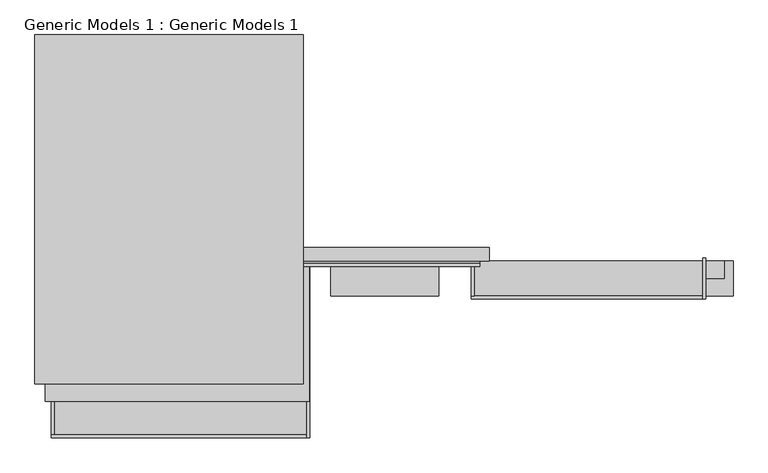
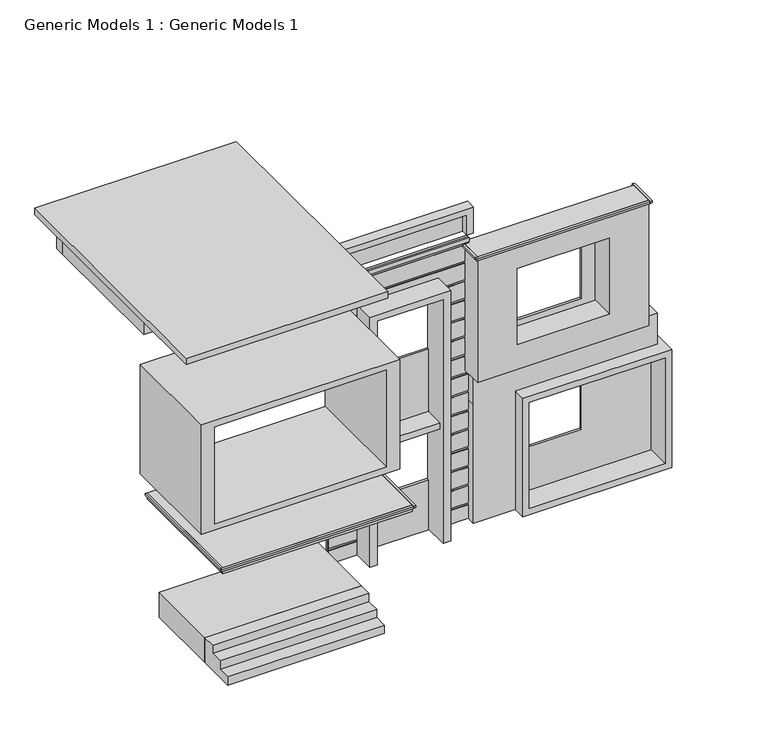
"""IFC4 building model written with IfcOpenShell, lengths in millimetres: proxy geometry, Generic Models 1 : Generic Models 1."""

from ifc_helpers import new_model, si_unit, frame, origin, origin_with_axes, place, context, project, spatial, polyline, outline, extrude, faceted_brep, source, transform, mapped, element, save


def generic_models_1_generic_models_1_556d1784(model_context):
    return source(origin(), model_context, "Body", "SolidModel", [
        extrude(outline(polyline([(-7879.4679297, 143.2196292), (-7879.4679297, -85.3803708), (-8317.6179297, -85.3803708), (-8317.6179297, 143.2196292), (-7879.4679297, 143.2196292)])), frame((0.0, 0.0, 7490.4399671), z_axis=(0.0, 0.0, 1.0), x_axis=(1.0, 0.0, 0.0)), (0.0, 0.0, 1.0), 202.0307064),
        extrude(outline(polyline([(-8031.8679297, 144.1522509), (-8031.8679297, 3685.9303652), (-7879.4679297, 3685.9303652), (-7879.4679297, 144.1522509), (-8031.8679297, 144.1522509)])), frame((0.0, 0.0, 6858.0), z_axis=(0.0, 0.0, 1.0), x_axis=(1.0, 0.0, 0.0)), (0.0, 0.0, 1.0), 834.4706735),
        extrude(outline(polyline([(-9568.5679297, 3838.3303652), (-9339.9679297, 3838.3303652), (-7879.4679297, 3838.3303652), (-7879.4679297, 3685.9303652), (-9339.9679297, 3685.9303652), (-9339.9679297, 3394.4196292), (-9568.5679297, 3394.4196292), (-11930.7679297, 3394.4196292), (-11930.7679297, 143.2196292), (-12159.3679297, 143.2196292), (-12159.3679297, 3394.4196292), (-12159.3679297, 3623.0196292), (-9568.5679297, 3623.0196292), (-9568.5679297, 3838.3303652)])), frame((0.0, 0.0, 6858.0), z_axis=(0.0, 0.0, 1.0), x_axis=(1.0, 0.0, 0.0)), (0.0, 0.0, 1.0), 834.4706735),
        extrude(outline(polyline([(-7879.4679297, -2224.2989686), (-12540.3679297, -2224.2989686), (-12540.3679297, 3838.3303652), (-7879.4679297, 3838.3303652), (-7879.4679297, -2224.2989686)])), frame((0.0, 0.0, 7692.4706735), z_axis=(0.0, 0.0, 1.0), x_axis=(1.0, 0.0, 0.0)), (0.0, 0.0, 1.0), 152.4),
        extrude(outline(polyline([(-8063.6179297, 143.2196292), (-4812.4179297, 143.2196292), (-4812.4179297, 79.7196292), (-8063.6179297, 79.7196292), (-8063.6179297, 143.2196292)])), frame((0.0, 0.0, 6858.0), z_axis=(0.0, 0.0, 1.0), x_axis=(1.0, 0.0, 0.0)), (0.0, 0.0, 1.0), 486.1154283),
        extrude(outline(polyline([(6858.0, -8063.6179297), (7344.1154283, -8063.6179297), (7344.1154283, -4812.4179297), (6858.0, -4812.4179297), (6858.0, -4660.0179297), (7496.5154283, -4660.0179297), (7496.5154283, -8298.5679297), (6858.0, -8298.5679297), (6858.0, -8063.6179297)])), frame((0.0, -85.3803708, 0.0), z_axis=(0.0, 1.0, 0.0), x_axis=(0.0, 0.0, 1.0)), (0.0, 0.0, 1.0), 228.6),
        extrude(outline(polyline([(-900.8179297, -34.5803708), (-900.8179297, -745.7803708), (-951.6179297, -745.7803708), (-951.6179297, -34.5803708), (-900.8179297, -34.5803708)])), frame((0.0, 0.0, 6680.2), z_axis=(0.0, 0.0, 1.0), x_axis=(1.0, 0.0, 0.0)), (0.0, 0.0, 1.0), 50.8),
        extrude(outline(polyline([(-4964.8179297, -694.9803708), (-4964.8179297, -186.9803708), (-4914.0179297, -186.9803708), (-4914.0179297, -694.9803708), (-4964.8179297, -694.9803708)])), frame((0.0, 0.0, 6680.2), z_axis=(0.0, 0.0, 1.0), x_axis=(1.0, 0.0, 0.0)), (0.0, 0.0, 1.0), 50.8),
        extrude(outline(polyline([(-951.6179297, -745.7803708), (-4964.8179297, -745.7803708), (-4964.8179297, -694.9803708), (-951.6179297, -694.9803708), (-951.6179297, -745.7803708)])), frame((0.0, 0.0, 6680.2), z_axis=(0.0, 0.0, 1.0), x_axis=(1.0, 0.0, 0.0)), (0.0, 0.0, 1.0), 50.8),
        extrude(outline(polyline([(4267.2, -4018.6679297), (4267.2, -1885.0679297), (6121.4, -1885.0679297), (6121.4, -4018.6679297), (4267.2, -4018.6679297)]), holes=[polyline([(4419.6, -3713.8679297), (5969.0, -3713.8679297), (5969.0, -2189.8679297), (4419.6, -2189.8679297), (4419.6, -3713.8679297)])]), frame((0.0, -136.1803708, 0.0), z_axis=(0.0, 1.0, 0.0), x_axis=(0.0, 0.0, 1.0)), (0.0, 0.0, 1.0), 50.8),
        extrude(outline(polyline([(1219.2, -2189.8679297), (1219.2, -3713.8679297), (152.4, -3713.8679297), (152.4, -2189.8679297), (152.4, -576.9679297), (2743.2, -576.9679297), (2743.2, -2189.8679297), (1219.2, -2189.8679297)])), frame((0.0, -136.1803708, 0.0), z_axis=(0.0, 1.0, 0.0), x_axis=(0.0, 0.0, 1.0)), (0.0, 0.0, 1.0), 50.8),
        extrude(outline(polyline([(3657.6, -4914.0179297), (3657.6, -951.6179297), (6731.0, -951.6179297), (6731.0, -4914.0179297), (3657.6, -4914.0179297)]), holes=[polyline([(6121.4, -1866.0179297), (4267.2, -1866.0179297), (4267.2, -3999.6179297), (6121.4, -3999.6179297), (6121.4, -1866.0179297)])]), frame((0.0, -694.9803708, 0.0), z_axis=(0.0, 1.0, 0.0), x_axis=(0.0, 0.0, 1.0)), (0.0, 0.0, 1.0), 609.6),
        extrude(outline(polyline([(2895.6, -4836.3153615), (0.0, -4836.3153615), (0.0, -3866.2679297), (2895.6, -3866.2679297), (2895.6, -576.9679297), (3657.6, -576.9679297), (3657.6, -4836.3153615), (2895.6, -4836.3153615)])), frame((0.0, -390.1803708, 0.0), z_axis=(0.0, 1.0, 0.0), x_axis=(0.0, 0.0, 1.0)), (0.0, 0.0, 1.0), 304.8),
        extrude(outline(polyline([(0.0, -3866.2679297), (0.0, -424.5679297), (2895.6, -424.5679297), (2895.6, -3866.2679297), (0.0, -3866.2679297)]), holes=[polyline([(152.4, -3713.8679297), (2743.2, -3713.8679297), (2743.2, -576.9679297), (152.4, -576.9679297), (152.4, -3713.8679297)])]), frame((0.0, -694.9803708, 0.0), z_axis=(0.0, 1.0, 0.0), x_axis=(0.0, 0.0, 1.0)), (0.0, 0.0, 1.0), 609.6),
        faceted_brep([(-8063.6179297, -186.9803708, 0.0), (-7409.7974608, -186.9803708, 0.0), (-7409.7974608, -186.9803708, 333.7154283), (-8063.6179297, -186.9803708, 333.7154283), (-7409.7974608, -186.9803708, 6121.4), (-5535.77405, -186.9803708, 6121.4), (-5535.77405, -186.9803708, 5870.9154283), (-4817.2653615, -186.9803708, 5870.9154283), (-4817.2653615, -186.9803708, 6277.3154283), (-8063.6179297, -186.9803708, 6277.3154283), (-8063.6179297, -186.9803708, 5870.9154283), (-7409.7974608, -186.9803708, 5870.9154283), (-5535.77405, -186.9803708, 0.0), (-4817.2653615, -186.9803708, 0.0), (-4817.2653615, -186.9803708, 333.7154283), (-5535.77405, -186.9803708, 333.7154283), (-4817.2653615, -186.9803708, 6858.0), (-8063.6179297, -186.9803708, 6858.0), (-8063.6179297, -186.9803708, 6759.9154283), (-4817.2653615, -186.9803708, 6759.9154283), (-7409.7974608, -186.9803708, 384.5154283), (-7409.7974608, -186.9803708, 790.9154283), (-8063.6179297, -186.9803708, 790.9154283), (-8063.6179297, -186.9803708, 384.5154283), (-7409.7974608, -186.9803708, 841.7154283), (-7409.7974608, -186.9803708, 1248.1154283), (-8063.6179297, -186.9803708, 1248.1154283), (-8063.6179297, -186.9803708, 841.7154283), (-7409.7974608, -186.9803708, 1298.9154283), (-7409.7974608, -186.9803708, 1705.3154283), (-8063.6179297, -186.9803708, 1705.3154283), (-8063.6179297, -186.9803708, 1298.9154283), (-7409.7974608, -186.9803708, 1756.1154283), (-7409.7974608, -186.9803708, 2162.5154283), (-8063.6179297, -186.9803708, 2162.5154283), (-8063.6179297, -186.9803708, 1756.1154283), (-7409.7974608, -186.9803708, 2213.3154283), (-7409.7974608, -186.9803708, 2619.7154283), (-8063.6179297, -186.9803708, 2619.7154283), (-8063.6179297, -186.9803708, 2213.3154283), (-7409.7974608, -186.9803708, 2670.5154283), (-7409.7974608, -186.9803708, 3076.9154283), (-7749.8885054, -186.9803708, 3076.9154283), (-7749.8885054, -186.9803708, 3127.7154283), (-7409.7974608, -186.9803708, 3127.7154283), (-7409.7974608, -186.9803708, 3534.1154283), (-7860.4179297, -186.9803708, 3534.1154283), (-7860.4179297, -186.9803708, 3584.9154283), (-7409.7974608, -186.9803708, 3584.9154283), (-7409.7974608, -186.9803708, 3991.3154283), (-8063.6179297, -186.9803708, 3991.3154283), (-8063.6179297, -186.9803708, 2670.5154283), (-7409.7974608, -186.9803708, 4042.1154283), (-7409.7974608, -186.9803708, 4448.5154283), (-8063.6179297, -186.9803708, 4448.5154283), (-8063.6179297, -186.9803708, 4042.1154283), (-7409.7974608, -186.9803708, 4499.3154283), (-7409.7974608, -186.9803708, 4905.7154283), (-8063.6179297, -186.9803708, 4905.7154283), (-8063.6179297, -186.9803708, 4499.3154283), (-7409.7974608, -186.9803708, 4956.5154283), (-7409.7974608, -186.9803708, 5362.9154283), (-8063.6179297, -186.9803708, 5362.9154283), (-8063.6179297, -186.9803708, 4956.5154283), (-7409.7974608, -186.9803708, 5413.7154283), (-7409.7974608, -186.9803708, 5820.1154283), (-8063.6179297, -186.9803708, 5820.1154283), (-8063.6179297, -186.9803708, 5413.7154283), (-5535.77405, -186.9803708, 790.9154283), (-5535.77405, -186.9803708, 384.5154283), (-4817.2653615, -186.9803708, 384.5154283), (-4817.2653615, -186.9803708, 790.9154283), (-5535.77405, -186.9803708, 1248.1154283), (-5535.77405, -186.9803708, 841.7154283), (-4817.2653615, -186.9803708, 841.7154283), (-4817.2653615, -186.9803708, 1248.1154283), (-5535.77405, -186.9803708, 1705.3154283), (-5535.77405, -186.9803708, 1298.9154283), (-4817.2653615, -186.9803708, 1298.9154283), (-4817.2653615, -186.9803708, 1705.3154283), (-5535.77405, -186.9803708, 2162.5154283), (-5535.77405, -186.9803708, 1756.1154283), (-4817.2653615, -186.9803708, 1756.1154283), (-4817.2653615, -186.9803708, 2162.5154283), (-5535.77405, -186.9803708, 2619.7154283), (-5535.77405, -186.9803708, 2213.3154283), (-4817.2653615, -186.9803708, 2213.3154283), (-4817.2653615, -186.9803708, 2619.7154283), (-5535.77405, -186.9803708, 3076.9154283), (-5535.77405, -186.9803708, 2670.5154283), (-4817.2653615, -186.9803708, 2670.5154283), (-4817.2653615, -186.9803708, 3076.9154283), (-5535.77405, -186.9803708, 3534.1154283), (-5535.77405, -186.9803708, 3127.7154283), (-4817.2653615, -186.9803708, 3127.7154283), (-4817.2653615, -186.9803708, 3534.1154283), (-5535.77405, -186.9803708, 3991.3154283), (-5535.77405, -186.9803708, 3584.9154283), (-4817.2653615, -186.9803708, 3584.9154283), (-4817.2653615, -186.9803708, 3991.3154283), (-5535.77405, -186.9803708, 4448.5154283), (-5535.77405, -186.9803708, 4042.1154283), (-4817.2653615, -186.9803708, 4042.1154283), (-4817.2653615, -186.9803708, 4448.5154283), (-5535.77405, -186.9803708, 4905.7154283), (-5535.77405, -186.9803708, 4499.3154283), (-4817.2653615, -186.9803708, 4499.3154283), (-4817.2653615, -186.9803708, 4905.7154283), (-5535.77405, -186.9803708, 5362.9154283), (-5535.77405, -186.9803708, 4956.5154283), (-4817.2653615, -186.9803708, 4956.5154283), (-4817.2653615, -186.9803708, 5362.9154283), (-5535.77405, -186.9803708, 5820.1154283), (-5535.77405, -186.9803708, 5413.7154283), (-4817.2653615, -186.9803708, 5413.7154283), (-4817.2653615, -186.9803708, 5820.1154283), (-4817.2653615, -186.9803708, 6328.1154283), (-4817.2653615, -186.9803708, 6709.1154283), (-8063.6179297, -186.9803708, 6709.1154283), (-8063.6179297, -186.9803708, 6328.1154283), (-8063.6179297, -136.1803708, 0.0), (-8063.6179297, -136.1803708, 6858.0), (-4817.2653615, -136.1803708, 6858.0), (-4817.2653615, -136.1803708, 0.0), (-5535.77405, -136.1803708, 0.0), (-5535.77405, -136.1803708, 6121.4), (-7409.7974608, -136.1803708, 6121.4), (-7409.7974608, -136.1803708, 0.0), (-7409.7974608, -174.2803708, 5870.9154283), (-7409.7974608, -174.2803708, 5820.1154283), (-7409.7974608, -174.2803708, 5413.7154283), (-7409.7974608, -174.2803708, 5362.9154283), (-7409.7974608, -174.2803708, 4956.5154283), (-7409.7974608, -174.2803708, 4905.7154283), (-7409.7974608, -174.2803708, 4499.3154283), (-7409.7974608, -174.2803708, 4448.5154283), (-7409.7974608, -174.2803708, 4042.1154283), (-7409.7974608, -174.2803708, 3991.3154283), (-7409.7974608, -174.2803708, 3584.9154283), (-7409.7974608, -174.2803708, 3534.1154283), (-7409.7974608, -174.2803708, 3127.7154283), (-7409.7974608, -174.2803708, 3076.9154283), (-7409.7974608, -174.2803708, 2670.5154283), (-7409.7974608, -174.2803708, 2619.7154283), (-7409.7974608, -174.2803708, 2213.3154283), (-7409.7974608, -174.2803708, 2162.5154283), (-7409.7974608, -174.2803708, 1756.1154283), (-7409.7974608, -174.2803708, 1705.3154283), (-7409.7974608, -174.2803708, 1298.9154283), (-7409.7974608, -174.2803708, 1248.1154283), (-7409.7974608, -174.2803708, 841.7154283), (-7409.7974608, -174.2803708, 790.9154283), (-7409.7974608, -174.2803708, 384.5154283), (-7409.7974608, -174.2803708, 333.7154283), (-5535.77405, -174.2803708, 333.7154283), (-5535.77405, -174.2803708, 384.5154283), (-5535.77405, -174.2803708, 790.9154283), (-5535.77405, -174.2803708, 841.7154283), (-5535.77405, -174.2803708, 1248.1154283), (-5535.77405, -174.2803708, 1298.9154283), (-5535.77405, -174.2803708, 1705.3154283), (-5535.77405, -174.2803708, 1756.1154283), (-5535.77405, -174.2803708, 2162.5154283), (-5535.77405, -174.2803708, 2213.3154283), (-5535.77405, -174.2803708, 2619.7154283), (-5535.77405, -174.2803708, 2670.5154283), (-5535.77405, -174.2803708, 3076.9154283), (-5535.77405, -174.2803708, 3127.7154283), (-5535.77405, -174.2803708, 3534.1154283), (-5535.77405, -174.2803708, 3584.9154283), (-5535.77405, -174.2803708, 3991.3154283), (-5535.77405, -174.2803708, 4042.1154283), (-5535.77405, -174.2803708, 4448.5154283), (-5535.77405, -174.2803708, 4499.3154283), (-5535.77405, -174.2803708, 4905.7154283), (-5535.77405, -174.2803708, 4956.5154283), (-5535.77405, -174.2803708, 5362.9154283), (-5535.77405, -174.2803708, 5413.7154283), (-5535.77405, -174.2803708, 5820.1154283), (-5535.77405, -174.2803708, 5870.9154283), (-4817.2653615, -174.2803708, 6759.9154283), (-4817.2653615, -174.2803708, 6709.1154283), (-4817.2653615, -174.2803708, 6328.1154283), (-4817.2653615, -174.2803708, 6277.3154283), (-4817.2653615, -174.2803708, 5870.9154283), (-4817.2653615, -174.2803708, 5820.1154283), (-4817.2653615, -174.2803708, 5413.7154283), (-4817.2653615, -174.2803708, 5362.9154283), (-4817.2653615, -174.2803708, 4956.5154283), (-4817.2653615, -174.2803708, 4905.7154283), (-4817.2653615, -174.2803708, 4499.3154283), (-4817.2653615, -174.2803708, 4448.5154283), (-4817.2653615, -174.2803708, 4042.1154283), (-4817.2653615, -174.2803708, 3991.3154283), (-4817.2653615, -174.2803708, 3584.9154283), (-4817.2653615, -174.2803708, 3534.1154283), (-4817.2653615, -174.2803708, 3127.7154283), (-4817.2653615, -174.2803708, 3076.9154283), (-4817.2653615, -174.2803708, 2670.5154283), (-4817.2653615, -174.2803708, 2619.7154283), (-4817.2653615, -174.2803708, 2213.3154283), (-4817.2653615, -174.2803708, 2162.5154283), (-4817.2653615, -174.2803708, 1756.1154283), (-4817.2653615, -174.2803708, 1705.3154283), (-4817.2653615, -174.2803708, 1298.9154283), (-4817.2653615, -174.2803708, 1248.1154283), (-4817.2653615, -174.2803708, 841.7154283), (-4817.2653615, -174.2803708, 790.9154283), (-4817.2653615, -174.2803708, 384.5154283), (-4817.2653615, -174.2803708, 333.7154283), (-8063.6179297, -174.2803708, 333.7154283), (-8063.6179297, -174.2803708, 384.5154283), (-8063.6179297, -174.2803708, 790.9154283), (-8063.6179297, -174.2803708, 841.7154283), (-8063.6179297, -174.2803708, 1248.1154283), (-8063.6179297, -174.2803708, 1298.9154283), (-8063.6179297, -174.2803708, 1705.3154283), (-8063.6179297, -174.2803708, 1756.1154283), (-8063.6179297, -174.2803708, 2162.5154283), (-8063.6179297, -174.2803708, 2213.3154283), (-8063.6179297, -174.2803708, 2619.7154283), (-8063.6179297, -174.2803708, 2670.5154283), (-8063.6179297, -174.2803708, 3991.3154283), (-8063.6179297, -174.2803708, 4042.1154283), (-8063.6179297, -174.2803708, 4448.5154283), (-8063.6179297, -174.2803708, 4499.3154283), (-8063.6179297, -174.2803708, 4905.7154283), (-8063.6179297, -174.2803708, 4956.5154283), (-8063.6179297, -174.2803708, 5362.9154283), (-8063.6179297, -174.2803708, 5413.7154283), (-8063.6179297, -174.2803708, 5820.1154283), (-8063.6179297, -174.2803708, 5870.9154283), (-8063.6179297, -174.2803708, 6277.3154283), (-8063.6179297, -174.2803708, 6328.1154283), (-8063.6179297, -174.2803708, 6709.1154283), (-8063.6179297, -174.2803708, 6759.9154283), (-7749.8885054, -174.2803708, 3127.7154283), (-7749.8885054, -174.2803708, 3076.9154283), (-7860.4179297, -174.2803708, 3584.9154283), (-7860.4179297, -174.2803708, 3534.1154283)], [[[0, 1, 2, 3]], [[4, 5, 6, 7, 8, 9, 10, 11]], [[12, 13, 14, 15]], [[16, 17, 18, 19]], [[20, 21, 22, 23]], [[24, 25, 26, 27]], [[28, 29, 30, 31]], [[32, 33, 34, 35]], [[36, 37, 38, 39]], [[40, 41, 42, 43, 44, 45, 46, 47, 48, 49, 50, 51]], [[52, 53, 54, 55]], [[56, 57, 58, 59]], [[60, 61, 62, 63]], [[64, 65, 66, 67]], [[68, 69, 70, 71]], [[72, 73, 74, 75]], [[76, 77, 78, 79]], [[80, 81, 82, 83]], [[84, 85, 86, 87]], [[88, 89, 90, 91]], [[92, 93, 94, 95]], [[96, 97, 98, 99]], [[100, 101, 102, 103]], [[104, 105, 106, 107]], [[108, 109, 110, 111]], [[112, 113, 114, 115]], [[116, 117, 118, 119]], [[120, 121, 122, 123, 124, 125, 126, 127]], [[1, 0, 120, 127]], [[127, 126, 4, 11, 128, 129, 65, 64, 130, 131, 61, 60, 132, 133, 57, 56, 134, 135, 53, 52, 136, 137, 49, 48, 138, 139, 45, 44, 140, 141, 41, 40, 142, 143, 37, 36, 144, 145, 33, 32, 146, 147, 29, 28, 148, 149, 25, 24, 150, 151, 21, 20, 152, 153, 2, 1]], [[5, 4, 126, 125]], [[125, 124, 12, 15, 154, 155, 69, 68, 156, 157, 73, 72, 158, 159, 77, 76, 160, 161, 81, 80, 162, 163, 85, 84, 164, 165, 89, 88, 166, 167, 93, 92, 168, 169, 97, 96, 170, 171, 101, 100, 172, 173, 105, 104, 174, 175, 109, 108, 176, 177, 113, 112, 178, 179, 6, 5]], [[13, 12, 124, 123]], [[123, 122, 16, 19, 180, 181, 117, 116, 182, 183, 8, 7, 184, 185, 115, 114, 186, 187, 111, 110, 188, 189, 107, 106, 190, 191, 103, 102, 192, 193, 99, 98, 194, 195, 95, 94, 196, 197, 91, 90, 198, 199, 87, 86, 200, 201, 83, 82, 202, 203, 79, 78, 204, 205, 75, 74, 206, 207, 71, 70, 208, 209, 14, 13]], [[17, 16, 122, 121]], [[121, 120, 0, 3, 210, 211, 23, 22, 212, 213, 27, 26, 214, 215, 31, 30, 216, 217, 35, 34, 218, 219, 39, 38, 220, 221, 51, 50, 222, 223, 55, 54, 224, 225, 59, 58, 226, 227, 63, 62, 228, 229, 67, 66, 230, 231, 10, 9, 232, 233, 119, 118, 234, 235, 18, 17]], [[152, 211, 210, 153]], [[150, 213, 212, 151]], [[148, 215, 214, 149]], [[146, 217, 216, 147]], [[144, 219, 218, 145]], [[142, 221, 220, 143]], [[140, 236, 237, 141]], [[138, 238, 239, 139]], [[136, 223, 222, 137]], [[134, 225, 224, 135]], [[132, 227, 226, 133]], [[130, 229, 228, 131]], [[128, 231, 230, 129]], [[182, 233, 232, 183]], [[180, 235, 234, 181]], [[208, 155, 154, 209]], [[206, 157, 156, 207]], [[204, 159, 158, 205]], [[202, 161, 160, 203]], [[200, 163, 162, 201]], [[198, 165, 164, 199]], [[196, 167, 166, 197]], [[194, 169, 168, 195]], [[192, 171, 170, 193]], [[190, 173, 172, 191]], [[188, 175, 174, 189]], [[186, 177, 176, 187]], [[184, 179, 178, 185]], [[153, 210, 3, 2]], [[211, 152, 20, 23]], [[151, 212, 22, 21]], [[213, 150, 24, 27]], [[149, 214, 26, 25]], [[215, 148, 28, 31]], [[147, 216, 30, 29]], [[217, 146, 32, 35]], [[145, 218, 34, 33]], [[219, 144, 36, 39]], [[143, 220, 38, 37]], [[221, 142, 40, 51]], [[141, 237, 42, 41]], [[237, 236, 43, 42]], [[236, 140, 44, 43]], [[139, 239, 46, 45]], [[239, 238, 47, 46]], [[238, 138, 48, 47]], [[137, 222, 50, 49]], [[223, 136, 52, 55]], [[135, 224, 54, 53]], [[225, 134, 56, 59]], [[133, 226, 58, 57]], [[227, 132, 60, 63]], [[131, 228, 62, 61]], [[229, 130, 64, 67]], [[129, 230, 66, 65]], [[231, 128, 11, 10]], [[183, 232, 9, 8]], [[233, 182, 116, 119]], [[181, 234, 118, 117]], [[235, 180, 19, 18]], [[209, 154, 15, 14]], [[155, 208, 70, 69]], [[207, 156, 68, 71]], [[157, 206, 74, 73]], [[205, 158, 72, 75]], [[159, 204, 78, 77]], [[203, 160, 76, 79]], [[161, 202, 82, 81]], [[201, 162, 80, 83]], [[163, 200, 86, 85]], [[199, 164, 84, 87]], [[165, 198, 90, 89]], [[197, 166, 88, 91]], [[167, 196, 94, 93]], [[195, 168, 92, 95]], [[169, 194, 98, 97]], [[193, 170, 96, 99]], [[171, 192, 102, 101]], [[191, 172, 100, 103]], [[173, 190, 106, 105]], [[189, 174, 104, 107]], [[175, 188, 110, 109]], [[187, 176, 108, 111]], [[177, 186, 114, 113]], [[185, 178, 112, 115]], [[179, 184, 7, 6]]]),
        extrude(outline(polyline([(0.0, -8063.6179297), (0.0, -7238.1179297), (6121.4, -7238.1179297), (6121.4, -5535.77405), (0.0, -5535.77405), (0.0, -4817.2653615), (6858.0, -4817.2653615), (6858.0, -8063.6179297), (0.0, -8063.6179297)])), frame((0.0, -136.1803708, 0.0), z_axis=(0.0, 1.0, 0.0), x_axis=(0.0, 0.0, 1.0)), (0.0, 0.0, 1.0), 50.8),
        extrude(outline(polyline([(5969.0, -5714.1179297), (0.0, -5714.1179297), (0.0, -5535.77405), (6121.4, -5535.77405), (6121.4, -7409.7974608), (0.0, -7409.7974608), (0.0, -7238.1179297), (5969.0, -7238.1179297), (5969.0, -5714.1179297)])), frame((0.0, -694.9803708, 0.0), z_axis=(0.0, 1.0, 0.0), x_axis=(0.0, 0.0, 1.0)), (0.0, 0.0, 1.0), 609.6),
        faceted_brep([(-12362.5679297, -2529.0989686, 6332.6526577), (-12362.5679297, -2529.0989686, 3657.6), (-7777.8679297, -2529.0989686, 3657.6), (-7777.8679297, -2529.0989686, 6332.6526577), (-12057.7679297, -2529.0989686, 3810.0), (-12057.7679297, -2529.0989686, 6180.2526577), (-8082.6679297, -2529.0989686, 6180.2526577), (-8082.6679297, -2529.0989686, 3810.0), (-12362.5679297, -85.3803708, 6332.6526577), (-7777.8679297, -85.3803708, 6332.6526577), (-7777.8679297, -85.3803708, 3657.6), (-12362.5679297, -85.3803708, 3657.6), (-12057.7679297, -85.3803708, 3810.0), (-8082.6679297, -85.3803708, 3810.0), (-8082.6679297, -85.3803708, 6180.2526577), (-12057.7679297, -85.3803708, 6180.2526577), (-7777.8679297, -174.2803708, 4042.1154283), (-7777.8679297, -174.2803708, 3991.3154283), (-7777.8679297, -186.9803708, 3991.3154283), (-7777.8679297, -186.9803708, 4042.1154283), (-7777.8679297, -174.2803708, 4499.3154283), (-7777.8679297, -174.2803708, 4448.5154283), (-7777.8679297, -186.9803708, 4448.5154283), (-7777.8679297, -186.9803708, 4499.3154283), (-7777.8679297, -174.2803708, 4956.5154283), (-7777.8679297, -174.2803708, 4905.7154283), (-7777.8679297, -186.9803708, 4905.7154283), (-7777.8679297, -186.9803708, 4956.5154283), (-7777.8679297, -174.2803708, 5413.7154283), (-7777.8679297, -174.2803708, 5362.9154283), (-7777.8679297, -186.9803708, 5362.9154283), (-7777.8679297, -186.9803708, 5413.7154283), (-7777.8679297, -174.2803708, 5870.9154283), (-7777.8679297, -174.2803708, 5820.1154283), (-7777.8679297, -186.9803708, 5820.1154283), (-7777.8679297, -186.9803708, 5870.9154283), (-7777.8679297, -174.2803708, 6328.1154283), (-7777.8679297, -174.2803708, 6277.3154283), (-7777.8679297, -186.9803708, 6277.3154283), (-7777.8679297, -186.9803708, 6328.1154283), (-8063.6179297, -174.2803708, 6328.1154283), (-8063.6179297, -174.2803708, 6277.3154283), (-8063.6179297, -174.2803708, 4042.1154283), (-8063.6179297, -174.2803708, 3991.3154283), (-8063.6179297, -174.2803708, 4499.3154283), (-8063.6179297, -174.2803708, 4448.5154283), (-8063.6179297, -174.2803708, 4956.5154283), (-8063.6179297, -174.2803708, 4905.7154283), (-8063.6179297, -174.2803708, 5413.7154283), (-8063.6179297, -174.2803708, 5362.9154283), (-8063.6179297, -174.2803708, 5870.9154283), (-8063.6179297, -174.2803708, 5820.1154283), (-8063.6179297, -186.9803708, 6277.3154283), (-8063.6179297, -186.9803708, 6328.1154283), (-8063.6179297, -186.9803708, 3991.3154283), (-8063.6179297, -186.9803708, 4042.1154283), (-8063.6179297, -186.9803708, 4448.5154283), (-8063.6179297, -186.9803708, 4499.3154283), (-8063.6179297, -186.9803708, 4905.7154283), (-8063.6179297, -186.9803708, 4956.5154283), (-8063.6179297, -186.9803708, 5362.9154283), (-8063.6179297, -186.9803708, 5413.7154283), (-8063.6179297, -186.9803708, 5820.1154283), (-8063.6179297, -186.9803708, 5870.9154283)], [[[0, 1, 2, 3], [4, 5, 6, 7]], [[8, 9, 10, 11], [12, 13, 14, 15]], [[5, 4, 12, 15]], [[6, 5, 15, 14]], [[7, 6, 14, 13]], [[4, 7, 13, 12]], [[1, 0, 8, 11]], [[2, 1, 11, 10]], [[3, 2, 10, 9], [16, 17, 18, 19], [20, 21, 22, 23], [24, 25, 26, 27], [28, 29, 30, 31], [32, 33, 34, 35], [36, 37, 38, 39]], [[0, 3, 9, 8]], [[40, 41, 37, 36]], [[42, 43, 17, 16]], [[44, 45, 21, 20]], [[46, 47, 25, 24]], [[48, 49, 29, 28]], [[50, 51, 33, 32]], [[52, 53, 39, 38]], [[54, 55, 19, 18]], [[56, 57, 23, 22]], [[58, 59, 27, 26]], [[60, 61, 31, 30]], [[62, 63, 35, 34]], [[43, 54, 18, 17]], [[55, 42, 16, 19]], [[45, 56, 22, 21]], [[57, 44, 20, 23]], [[47, 58, 26, 25]], [[59, 46, 24, 27]], [[49, 60, 30, 29]], [[61, 48, 28, 31]], [[51, 62, 34, 33]], [[63, 50, 32, 35]], [[41, 52, 38, 37]], [[41, 40, 53, 52]], [[53, 40, 36, 39]], [[43, 42, 55, 54]], [[45, 44, 57, 56]], [[47, 46, 59, 58]], [[49, 48, 61, 60]], [[51, 50, 63, 62]]]),
        extrude(outline(polyline([(-7768.9385054, -85.3803708), (-7768.9385054, -3158.8511799), (-7819.7385054, -3158.8511799), (-7819.7385054, -85.3803708), (-7768.9385054, -85.3803708)])), frame((0.0, 0.0, 3086.5208873), z_axis=(0.0, 0.0, 1.0), x_axis=(1.0, 0.0, 0.0)), (0.0, 0.0, 1.0), 50.8),
        extrude(outline(polyline([(-5733.1679297, -593.3803708), (-7257.1679297, -593.3803708), (-7257.1679297, -136.1803708), (-5733.1679297, -136.1803708), (-5733.1679297, -593.3803708)])), frame((0.0, 0.0, 2743.2), z_axis=(0.0, 0.0, 1.0), x_axis=(1.0, 0.0, 0.0)), (0.0, 0.0, 1.0), 152.4),
        extrude(outline(polyline([(-5733.1679297, -136.1803708), (-7257.1679297, -136.1803708), (-7257.1679297, -85.3803708), (-5733.1679297, -85.3803708), (-5733.1679297, -136.1803708)])), frame((0.0, 0.0, 2895.6), z_axis=(0.0, 0.0, 1.0), x_axis=(1.0, 0.0, 0.0)), (0.0, 0.0, 1.0), 1524.0),
        extrude(outline(polyline([(-5733.1679297, -136.1803708), (-7257.1679297, -136.1803708), (-7257.1679297, -85.3803708), (-5733.1679297, -85.3803708), (-5733.1679297, -136.1803708)])), origin_with_axes(), (0.0, 0.0, 1.0), 1219.2),
        extrude(outline(polyline([(-5714.1179297, -136.1803708), (-7238.1179297, -136.1803708), (-7238.1179297, -85.3803708), (-5714.1179297, -85.3803708), (-5714.1179297, -136.1803708)])), frame((0.0, 0.0, 2743.2), z_axis=(0.0, 0.0, 1.0), x_axis=(1.0, 0.0, 0.0)), (0.0, 0.0, 1.0), 152.4),
        extrude(outline(polyline([(-7819.7385054, -3158.8511799), (-12255.0398919, -3158.8511799), (-12255.0398919, -3108.0511799), (-7819.7385054, -3108.0511799), (-7819.7385054, -3158.8511799)])), frame((0.0, 0.0, 3086.5208873), z_axis=(0.0, 0.0, 1.0), x_axis=(1.0, 0.0, 0.0)), (0.0, 0.0, 1.0), 50.8),
        extrude(outline(polyline([(-12255.0398919, -3108.0511799), (-12255.0398919, -85.4511799), (-12204.2398919, -85.4511799), (-12204.2398919, -3108.0511799), (-12255.0398919, -3108.0511799)])), frame((0.0, 0.0, 3086.5208873), z_axis=(0.0, 0.0, 1.0), x_axis=(1.0, 0.0, 0.0)), (0.0, 0.0, 1.0), 50.8),
        extrude(outline(polyline([(-7819.7385054, -3108.0511799), (-12204.2398919, -3108.0511799), (-12204.2398919, -85.3803708), (-7819.7385054, -85.3803708), (-7819.7385054, -3108.0511799)])), frame((0.0, 0.0, 2984.9208873), z_axis=(0.0, 0.0, 1.0), x_axis=(1.0, 0.0, 0.0)), (0.0, 0.0, 1.0), 152.4),
        extrude(outline(polyline([(-1919.4989686, 609.6), (-1919.4989686, 0.0), (-2833.8989686, 0.0), (-2833.8989686, 203.2), (-2529.0989686, 203.2), (-2529.0989686, 406.4), (-2224.2989686, 406.4), (-2224.2989686, 609.6), (-1919.4989686, 609.6)])), frame((-11930.7679297, 0.0, 0.0), z_axis=(1.0, 0.0, 0.0), x_axis=(0.0, 1.0, 0.0)), (0.0, 0.0, 1.0), 3619.5),
        extrude(outline(polyline([(-8311.2679297, -1919.4989686), (-11930.7679297, -1919.4989686), (-11930.7679297, -85.3803708), (-8311.2679297, -85.3803708), (-8311.2679297, -1919.4989686)])), origin_with_axes(), (0.0, 0.0, 1.0), 609.6),
    ])


if __name__ == "__main__":
    model = new_model("IFC4")
    model_context = context("Model", 3, world=origin())
    ifc_project = project(units=[si_unit("LENGTHUNIT", "METRE", prefix="MILLI")], contexts=[model_context])
    site = spatial("IfcSite", under=ifc_project)
    building = spatial("IfcBuilding", under=site)
    placement = place(None, origin())
    generic_models_1_generic_models_1_shape = generic_models_1_generic_models_1_556d1784(model_context)
    element("IfcBuildingElementProxy", 1, Name="Generic Models 1 : Generic Models 1", ObjectType="Generic Models 1 : Generic Models 1", at=placement, inside=building, context=model_context, shape_type="MappedRepresentation", body=[
        mapped(generic_models_1_generic_models_1_shape, transform((0.0, 0.0, 0.0), x_axis=(1.0, 0.0, 0.0), y_axis=(0.0, 1.0, 0.0), z_axis=(0.0, 0.0, 1.0))),
    ])
    save(model, "model.ifc")

# Revit data of these elements
# Element 1 (IfcBuildingElementProxy, "Generic Models 1 : Generic Models 1")
#   Materials on its faces: "light ash colour", "Laminate, Ivory, Matte", "Gypsum Wall Board", "Ash colour", "door colour", "window brick", "Ash brick", "Earth", "Concrete, Lightweight"
# Materials
#   "light ash colour": class "Generic", colour RGB 120 120 120, transparency 0, Cost = 0
#   "Laminate, Ivory, Matte": class "Plastic", colour RGB 247 247 239, transparency 0, Description = "Plastic Laminate - Ivory, Matte", Cost = 0
#   "Gypsum Wall Board": class "Generic", colour RGB 127 127 127, transparency 0, Description = "Gypsum Wall Board", Cost = 0
#   "Ash colour": class "Generic", colour RGB 120 120 120, transparency 0, Cost = 0
#   "door colour": class "Generic", colour RGB 120 120 120, transparency 0, Cost = 0
#   "window brick": class "Generic", colour RGB 120 120 120, transparency 0, Cost = 0
#   "Ash brick": class "Generic", colour RGB 120 120 120, transparency 0, Cost = 0
#   "Earth": class "Generic", colour RGB 97 75 62, transparency 0, Description = "Soil", Cost = 0
#   "Concrete, Lightweight": class "Concrete", colour RGB 142 141 140, transparency 0, Description = "Lightweight concrete", Cost = 0
